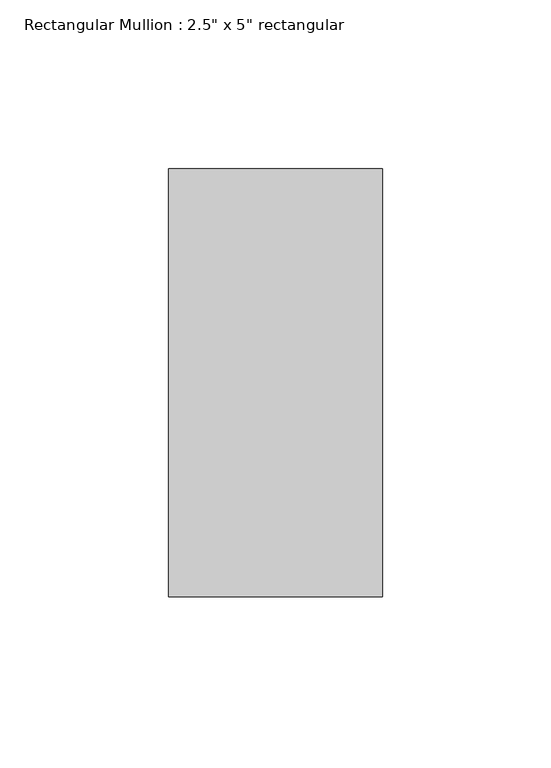
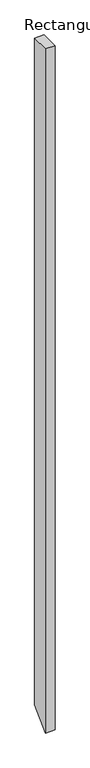
"""IFC4 building model written with IfcOpenShell, lengths in millimetres: member geometry."""

from ifc_helpers import new_model, si_unit, frame, origin, place, context, project, spatial, polyline, outline, extrude, source, transform, mapped, element, save


def member_ff8123a6(model_context):
    return source(origin(), model_context, "Body", "SweptSolid", [
        extrude(outline(polyline([(-63.5, 0.0), (63.5, 0.0), (63.5, -4758.2018512), (-63.5, -4885.2018512), (-63.5, 0.0)])), frame((-63.5, 0.0, 0.0), z_axis=(1.0, 0.0, 0.0), x_axis=(0.0, 1.0, 0.0)), (0.0, 0.0, 1.0), 63.5),
    ])


if __name__ == "__main__":
    model = new_model("IFC4")
    model_context = context("Model", 3, world=origin())
    ifc_project = project(units=[si_unit("LENGTHUNIT", "METRE", prefix="MILLI")], contexts=[model_context])
    site = spatial("IfcSite", under=ifc_project)
    building = spatial("IfcBuilding", under=site)
    placement = place(None, origin())
    member_shape = member_ff8123a6(model_context)
    element("IfcMember", 1, ObjectType="Rectangular Mullion : 2.5\" x 5\" rectangular", at=placement, inside=building, context=model_context, shape_type="MappedRepresentation", body=[
        mapped(member_shape, transform((0.0, 0.0, 0.0), x_axis=(1.0, 0.0, 0.0), y_axis=(0.0, 1.0, 0.0), z_axis=(0.0, 0.0, 1.0))),
    ])
    save(model, "model.ifc")

# Revit data of these elements
# Type "Rectangular Mullion : 2.5\" x 5\" rectangular"
#   built-in parameter 1007304 = 0.416667 (stored number, unit not read)
#   built-in parameter 1007301 = 0.104167 (stored number, unit not read)
#   built-in parameter 1007300 = 0.104167 (stored number, unit not read)
# Element 1 (IfcMember, "Rectangular Mullion : 2.5\" x 5\" rectangular")
#   Materials on its faces: "Aluminum"
# Materials
#   "Aluminum": class "Metal", colour RGB 247 247 247, transparency 0, Description = "Aluminum 6061", Cost = 0
